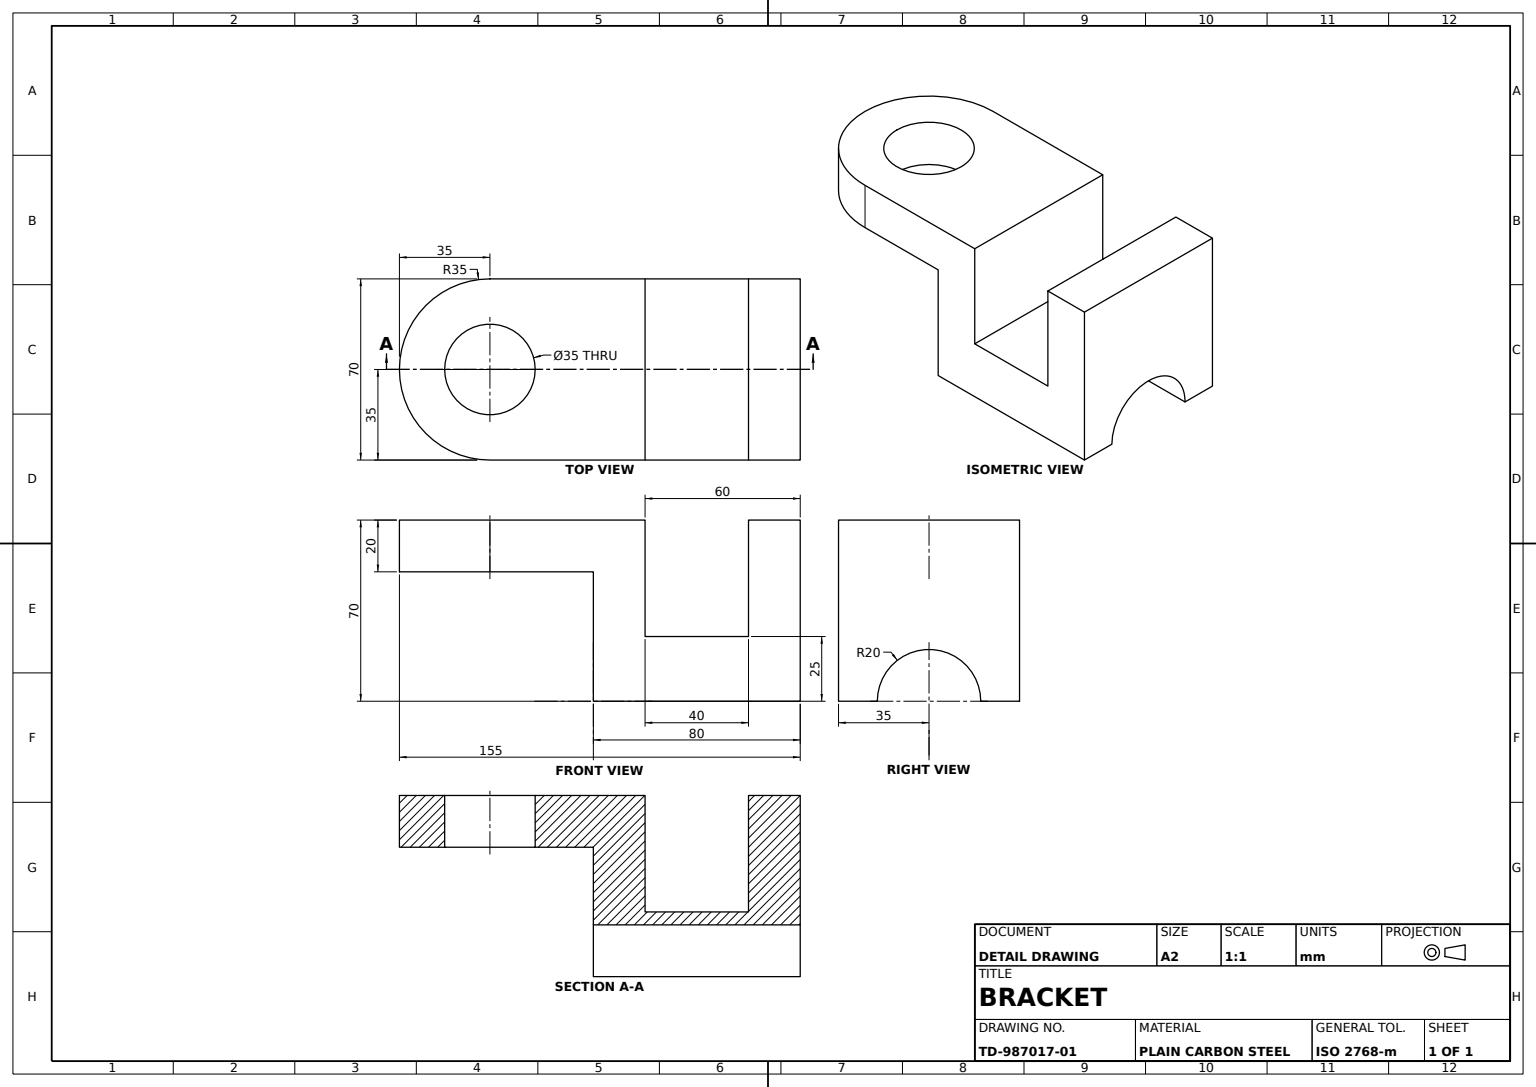
SolidWorks part; units mm, degrees
material "Plain Carbon Steel"
ref_plane "Front Plane" through (0, 0, 0) normal (0, 0, 1) x (1, 0, 0)
ref_plane "Top Plane" through (0, 0, 0) normal (0, 1, 0) x (1, 0, 0)
ref_plane "Right Plane" through (0, 0, 0) normal (1, 0, 0) x (0, 0, -1)
sketch "Base Block Sketch" plane through (0, 0, 0) normal (0, 0, 1) x (1, 0, 0)
  line L0 (0, 0) -> (70, 0)
  line L1 (70, 0) -> (70, -70)
  line L2 (70, -70) -> (0, -70)
  line L3 (0, -70) -> (0, 0)
  dimension "D1" = 70
extrude "Base Block" add sketch "Base Block Sketch" along normal blind 20
sketch "Step Block Sketch" plane through (0, -70, 0) normal (0, -1, 0) x (1, 0, 0)
  line L0 (0, 20) -> (0, 60)
  line L1 (0, 60) -> (70, 60)
  line L2 (70, 60) -> (70, 20)
  line L3 (70, 20) -> (0, 20)
  line L5 (0, 0) -> (70, 0) construction
  dimension "D1" = 60
extrude "Step Block" add sketch "Step Block Sketch" against normal blind 25
sketch "Upper Block Sketch" plane through (0, 0, 60) normal (0, 0, 1) x (1, 0, 0)
  line L0 (0, -45) -> (0, 0)
  line L1 (0, 0) -> (70, 0)
  line L2 (70, 0) -> (70, -45)
  line L3 (70, -45) -> (0, -45)
extrude "Upper Block" add sketch "Upper Block Sketch" along normal blind 20 separate body
sketch "Upright Wall Sketch" plane through (0, 0, 0) normal (-1, 0, 0) x (0, 0, 1)
  line L0 (60, -45) -> (80, -45)
  line L1 (80, -45) -> (80, -70)
  line L2 (80, -70) -> (60, -70)
  line L3 (60, -70) -> (60, -45)
  line L4 (0, 0) -> (0, -70) construction
  dimension "D1" = 80
extrude "Upright Wall" add sketch "Upright Wall Sketch" against normal blind 70
sketch "Arc Relief Cut Sketch" plane through (0, 0, 80) normal (0, 0, 1) x (1, 0, 0)
  line L0 (70, -70) -> (0, -70) construction
  line L1 (15, -70) -> (55, -70)
  arc A0 (55, -70) -> (15, -70) centre (35, -70) ccw
  dimension "D1" = 40
  dimension "D2" = 20
extrude "Arc Relief Cut" cut sketch "Arc Relief Cut Sketch" against normal blind 80
sketch "Rounded Lug Sketch" plane through (0, 0, 0) normal (0, 1, 0) x (1, 0, 0)
  line L0 (0, -80) -> (70, -80)
  line L2 (0, -80) -> (0, -120)
  line L3 (70, -80) -> (70, -120)
  line L4 (70, -60) -> (0, -60) construction
  arc A0 (0, -120) -> (70, -120) centre (35, -120) ccw
  dimension "D1" = 70
  dimension "D2" = 60
extrude "Rounded Lug" add sketch "Rounded Lug Sketch" against normal blind 20
sketch "Lug Hole Sketch" plane through (0, -20, 0) normal (0, -1, 0) x (1, 0, 0)
  circle A0 centre (35, 120) radius 17.5
  dimension "D1" = 35
  dimension "D2" = 35
extrude "Lug Hole" cut sketch "Lug Hole Sketch" against normal blind 20
